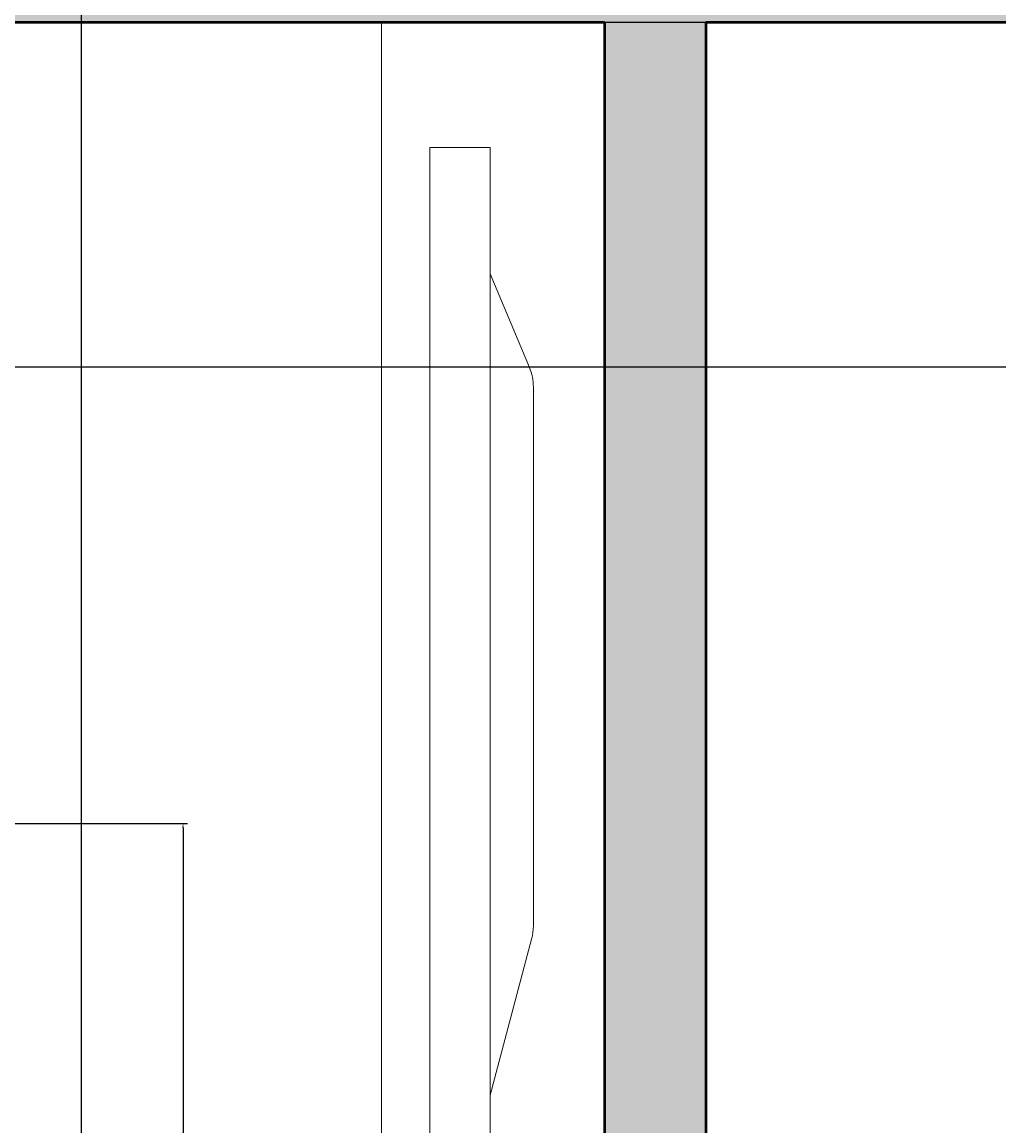
# Model space of a CAD drawing. Units: inches. Extents: x 2231 to 2461, y 2045 to 2455.
# Tile 86 of 95: x 2346 to 2384, y 2383 to 2427. Entities that reach past the tile are written whole.
import ezdxf

# ---------------------------------------------------------------- set-up
doc = ezdxf.new("R2010")
doc.units = ezdxf.units.IN
for name, color, linetype, lineweight in [('A-ANNO-DIMS', 2, 'Continuous', 18), ('A-EQPM', 8, 'Continuous', 18), ('A-FURN', 9, 'Continuous', 18), ('A-WALL', 7, 'Continuous', 50)]:
    doc.layers.add(name, color=color, linetype=linetype, lineweight=lineweight)
doc.layers.add('A-WALL-PATT', color=18, linetype='Continuous', lineweight=13, true_color=0x000000)
doc.styles.get("Standard").update_dxf_attribs({"font": 'arial.ttf'})
doc.dimstyles.get("Standard").update_dxf_attribs({"dimtxt": 0.18, "dimasz": 0.18, "dimexe": 0.18, "dimexo": 0.0625, "dimgap": 0.09, "dimtad": 0, "dimtih": 1, "dimtoh": 1, "dimdec": 4, "dimzin": 0, "dimdsep": 46, "dimtxsty": 'Standard', "dimcen": 0.09, "dimadec": 0, "dimazin": 0, "dimtfac": 1, "dimtdec": 4, "dimtofl": 0, "dimtmove": 0, "dimatfit": 3, "dimfxl": 1, "dimtolj": 1, "dimtzin": 0, "dimarcsym": 0})

# ---------------------------------------------------------------- blocks, each defined once
blk = doc.blocks.new('*D20')
at = {"layer": 'A-ANNO-DIMS', "color": 0, "lineweight": -2, "transparency": 16777216}
for p, q in [((2340.251, 2395.253), (2352.368, 2395.253)), ((2352.188, 2395.073), (2352.188, 2365.435)), ((2352.188, 2335.433), (2352.188, 2365.071)), ((2340.251, 2335.253), (2352.368, 2335.253))]:
    blk.add_line(p, q, dxfattribs=at)
at = {"layer": 'A-ANNO-DIMS', "color": 0, "transparency": 16777216}
for points in [[(2352.158, 2395.073), (2352.218, 2395.073), (2352.188, 2395.253)], [(2352.158, 2335.433), (2352.218, 2335.433), (2352.188, 2335.253)]]:
    blk.add_solid(points, dxfattribs=at)
at = {"layer": 'Defpoints', "color": 0, "transparency": 16777216}
for p in [(2340.188, 2395.253), (2352.188, 2395.253), (2340.188, 2335.253)]:
    blk.add_point(p, dxfattribs=at)
at = {"layer": 'A-ANNO-DIMS', "color": 0, "transparency": 16777216, "insert": (2352.188, 2365.253), "char_height": 0.18, "attachment_point": 5}
blk.add_mtext('\\A1;60', dxfattribs=at)
blk = doc.blocks.new('*D66')
at = {"layer": 'A-ANNO-DIMS', "color": 0, "lineweight": -2, "transparency": 16777216}
for p, q in [((2348.189, 2096.895), (2348.189, 2454.645)), ((2408.794, 2096.895), (2408.794, 2454.645)), ((2348.369, 2454.465), (2378.167, 2454.465)), ((2408.614, 2454.465), (2378.815, 2454.465))]:
    blk.add_line(p, q, dxfattribs=at)
at = {"layer": 'A-ANNO-DIMS', "color": 0, "transparency": 16777216}
for points in [[(2348.369, 2454.495), (2348.369, 2454.435), (2348.189, 2454.465)], [(2408.614, 2454.495), (2408.614, 2454.435), (2408.794, 2454.465)]]:
    blk.add_solid(points, dxfattribs=at)
at = {"layer": 'Defpoints', "color": 0, "transparency": 16777216}
for p in [(2408.794, 2454.465), (2348.189, 2096.833), (2408.794, 2096.833)]:
    blk.add_point(p, dxfattribs=at)
at = {"layer": 'A-ANNO-DIMS', "color": 0, "transparency": 16777216, "insert": (2378.491, 2454.465), "char_height": 0.18, "attachment_point": 5}
blk.add_mtext('\\A1;60.6', dxfattribs=at)
blk = doc.blocks.new('*D68')
at = {"layer": 'A-ANNO-DIMS', "color": 0, "lineweight": -2, "transparency": 16777216}
for p, q in [((2285.882, 2426.833), (2460.606, 2426.833)), ((2460.426, 2426.653), (2460.426, 2420.225)), ((2460.426, 2413.433), (2460.426, 2419.861)), ((2278.251, 2413.253), (2460.606, 2413.253))]:
    blk.add_line(p, q, dxfattribs=at)
at = {"layer": 'A-ANNO-DIMS', "color": 0, "transparency": 16777216}
for points in [[(2460.396, 2426.653), (2460.456, 2426.653), (2460.426, 2426.833)], [(2460.396, 2413.433), (2460.456, 2413.433), (2460.426, 2413.253)]]:
    blk.add_solid(points, dxfattribs=at)
at = {"layer": 'Defpoints', "color": 0, "transparency": 16777216}
for p in [(2285.82, 2426.833), (2460.426, 2426.833), (2278.188, 2413.253)]:
    blk.add_point(p, dxfattribs=at)
at = {"layer": 'A-ANNO-DIMS', "color": 0, "transparency": 16777216, "insert": (2460.426, 2420.043), "char_height": 0.18, "attachment_point": 5}
blk.add_mtext('\\A1;13.58', dxfattribs=at)

msp = doc.modelspace()

# ---------------------------------------------------------------- hatches: boundary and pattern name
at = {"layer": 'A-WALL-PATT'}
h = msp.add_hatch(color=256, dxfattribs=at)
h.dxf.hatch_style = 1
h.paths.add_polyline_path([(2441.7935, 2269.1535), (2432.7935, 2269.1535), (2432.7935, 2186.8328), (2396.7935, 2186.8328), (2396.7935, 2286.8328), (2394.7935, 2286.8328), (2394.7935, 2186.8328), (2334.7935, 2186.8328), (2334.7935, 2182.8328), (2432.7935, 2182.8328), (2432.7935, 2072.8328), (2416.6639, 2072.8328), (2416.6639, 2063.8328), (2441.7935, 2063.8328)])
h.paths.add_polyline_path([(2368.6639, 2072.8328), (2367.04, 2072.8328), (2330.7942, 2072.8328), (2330.7397, 2063.8328), (2368.6639, 2063.8328)])
h.paths.add_polyline_path([(2300.7392, 2068.3328), (2300.7392, 2072.8328), (2298.7935, 2072.8328), (2294.7935, 2072.8328), (2258.7935, 2072.8328), (2258.7935, 2120.8328), (2294.7935, 2120.8328), (2298.7935, 2120.8328), (2298.7935, 2128.8328), (2294.7935, 2128.8328), (2294.7935, 2124.8328), (2258.7935, 2124.8328), (2258.7935, 2182.8328), (2294.7935, 2182.8328), (2294.7935, 2174.8328), (2298.7935, 2174.8328), (2298.7935, 2182.8328), (2304.7935, 2182.8328), (2304.7935, 2186.8328), (2258.7935, 2186.8328), (2258.7935, 2221.999), (2249.7935, 2221.999), (2249.7935, 2063.8328), (2300.7392, 2063.8328)])
h.paths.add_polyline_path([(2391.9338, 2435.8328), (2333.82, 2435.8328), (2333.82, 2426.8328), (2368.7935, 2426.8328), (2368.7935, 2374.9508), (2368.7935, 2370.8328), (2372.3935, 2370.8328), (2372.7935, 2370.8328), (2372.7935, 2426.8328), (2391.9338, 2426.8328)])
h.paths.add_polyline_path([(2441.7935, 2435.8328), (2415.9338, 2435.8328), (2415.9338, 2426.8328), (2432.7935, 2426.8328), (2432.7935, 2334.8328), (2372.7935, 2334.8328), (2372.7935, 2346.8328), (2368.7935, 2346.8328), (2368.7935, 2306.8328), (2360.7935, 2306.8328), (2360.7935, 2302.8328), (2368.7935, 2302.8328), (2372.7935, 2302.8328), (2372.7935, 2330.8328), (2432.7935, 2330.8328), (2432.7935, 2317.1535), (2441.7935, 2317.1535)])
h.paths.add_polyline_path([(2285.82, 2435.8328), (2249.7935, 2435.8328), (2249.7935, 2269.999), (2258.7935, 2269.999), (2258.7935, 2302.8328), (2318.8168, 2302.8328), (2330.7935, 2302.8328), (2330.7935, 2306.8328), (2258.7935, 2306.8328), (2258.7935, 2426.8328), (2285.82, 2426.8328)])

# ---------------------------------------------------------------- linework, layer by layer
at = {"layer": 'A-EQPM'}
msp.add_lwpolyline([(2361.91, 2421.8956), (2364.2888, 2421.8956), (2364.2888, 2380.0244), (2361.91, 2380.0244)], close=True, dxfattribs=at)
msp.add_lwpolyline([(2364.2888, 2416.9185), (2365.838, 2413.2215, -0.0995279), (2365.9934, 2412.4485), (2365.9934, 2391.2157, -0.06517), (2365.926, 2390.7009), (2364.2888, 2384.5544)], format="xyb", dxfattribs=at)
msp.add_lwpolyline([(2364.2888, 2384.5544), (2364.2888, 2416.9185)], dxfattribs=at)
at = {"layer": 'A-FURN'}
msp.add_lwpolyline([(2368.7935, 2426.8328), (2360.0091, 2426.8328), (2360.0091, 2374.9508), (2368.7935, 2374.9508)], close=True, dxfattribs=at)
at = {"layer": 'A-WALL'}
for p, q in [((2258.7935, 2426.8328), (2368.7935, 2426.8328)), ((2368.7935, 2426.8328), (2368.7935, 2370.8328)), ((2372.7935, 2426.8328), (2372.7935, 2370.8328)), ((2372.7935, 2426.8328), (2432.7935, 2426.8328))]:
    msp.add_line(p, q, dxfattribs=at)

# ---------------------------------------------------------------- dimensions: what is measured, and where the dimension line sits
at = {"layer": 'A-ANNO-DIMS'}
dim = msp.add_linear_dim(base=(2408.7935, 2454.4653), p1=(2348.1888, 2096.8328), p2=(2408.7935, 2096.8328), dimstyle='Standard', override={"dimdec": 1, "dimlfac": 1, "dimrnd": 0, "dimzin": 0, "dimdsep": 46, "dimlunit": 2}, dxfattribs=at)
dim.commit()
dim.dimension.update_dxf_attribs({"geometry": '*D66', "text_midpoint": (2378.4912, 2454.4653)})
for base, p1, p2, override, picture, middle in [((2460.426, 2426.8328), (2278.1881, 2413.2534), (2285.82, 2426.8328), {"dimdec": 2, "dimlfac": 1, "dimrnd": 0, "dimzin": 0, "dimdsep": 46, "dimlunit": 2}, '*D68', (2460.426, 2420.0431)), ((2352.1882, 2395.2534), (2340.1882, 2335.2534), (2340.1882, 2395.2534), {"dimdec": 0, "dimlfac": 1, "dimrnd": 0, "dimzin": 0, "dimdsep": 46, "dimlunit": 2}, '*D20', (2352.1882, 2365.2534))]:
    dim = msp.add_linear_dim(base=base, p1=p1, p2=p2, angle=90, dimstyle='Standard', override=override, dxfattribs=at)
    dim.commit()
    dim.dimension.update_dxf_attribs({"geometry": picture, "text_midpoint": middle})

doc.saveas('drawing.dxf')
